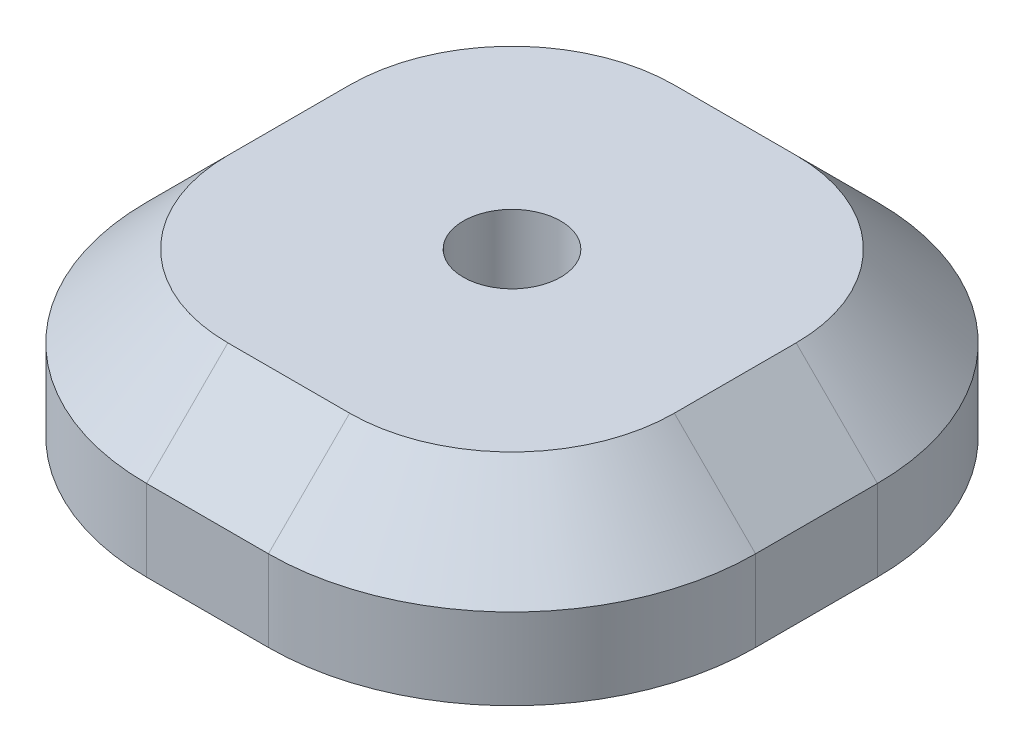
from build123d import *

# Parameters (mm, degrees)
BASE_PROFILE_SKETCH_75X75_W    = 75
BASE_PROFILE_SKETCH_75X75_H    = 75
BASE_BLOCK_75X75X20_DEPTH      = 20
CORNER_FILLETS_R30_R           = 30
TOP_EDGE_CHAMFER_10X45DEG_SIZE = 10
DOWEL_HOLE_A_12X10_D           = 12
DOWEL_HOLE_A_12X10_DEPTH       = 10
DOWEL_HOLE_A_12X10_TIP         = 3.605163714
DOWEL_HOLE_B_12X10_D           = 12
DOWEL_HOLE_B_12X10_DEPTH       = 10
DOWEL_HOLE_B_12X10_TIP         = 3.605163714


with BuildPart() as part:
    # Base Profile Sketch 75x75 → Base Block 75x75x20 (new body)
    with BuildSketch(Plane(origin=(0, 0, 0), x_dir=(1, 0, 0), z_dir=(0, 1, 0))):
        Rectangle(BASE_PROFILE_SKETCH_75X75_W, BASE_PROFILE_SKETCH_75X75_H)
    extrude(amount=BASE_BLOCK_75X75X20_DEPTH)

    # Corner Fillets R30
    corner_fillets_r30_edges = [part.edges().sort_by_distance(p)[0] for p in [
        (37.5, 10, 37.5),
        (-37.5, 10, 37.5),
        (-37.5, 10, -37.5),
        (37.5, 10, -37.5),
    ]]
    fillet(corner_fillets_r30_edges, radius=CORNER_FILLETS_R30_R)

    # Top Edge Chamfer 10x45deg
    top_edge_chamfer_10x45deg_edges = [part.edges().sort_by_distance(p)[0] for p in [
        (-37.5, 20, 0),
        (0, 20, -37.5),
        (37.5, 20, 0),
        (0, 20, 37.5),
        (-28.713203436, 20, 28.713203436),
        (28.713203436, 20, 28.713203436),
        (28.713203436, 20, -28.713203436),
        (-28.713203436, 20, -28.713203436),
    ]]
    chamfer(top_edge_chamfer_10x45deg_edges, length=TOP_EDGE_CHAMFER_10X45DEG_SIZE)

    # Dowel Hole A Ø12x10
    with Locations(Plane.ZX.offset(20)):
        with Locations((0, 0)):
            Hole(DOWEL_HOLE_A_12X10_D / 2, depth=DOWEL_HOLE_A_12X10_DEPTH)
            with Locations((0, 0, -(DOWEL_HOLE_A_12X10_DEPTH + DOWEL_HOLE_A_12X10_TIP / 2))):  # 118° drill point
                Cone(0, DOWEL_HOLE_A_12X10_D / 2, DOWEL_HOLE_A_12X10_TIP, mode=Mode.SUBTRACT)

    # Dowel Hole B Ø12x10
    with Locations(Plane(origin=(-12.5, 0, 12.5), x_dir=(0, 0, -1), z_dir=(0, -1, 0))):
        with Locations((0, 0), (0, 25), (25, 25), (25, 0)):
            Hole(DOWEL_HOLE_B_12X10_D / 2, depth=DOWEL_HOLE_B_12X10_DEPTH)
            with Locations((0, 0, -(DOWEL_HOLE_B_12X10_DEPTH + DOWEL_HOLE_B_12X10_TIP / 2))):  # 118° drill point
                Cone(0, DOWEL_HOLE_B_12X10_D / 2, DOWEL_HOLE_B_12X10_TIP, mode=Mode.SUBTRACT)


solid = part.part
